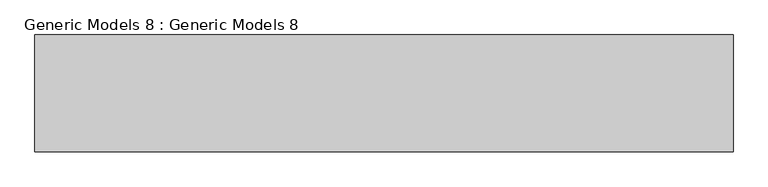
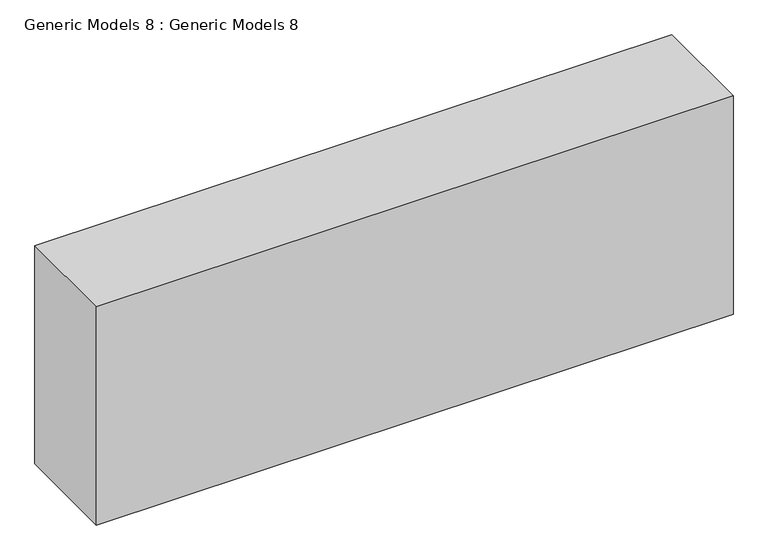
"""IFC4 building model written with IfcOpenShell, lengths in millimetres: proxy geometry, Generic Models 8 : Generic Models 8."""

from ifc_helpers import new_model, si_unit, frame, origin, place, context, project, spatial, polyline, outline, extrude, source, transform, mapped, element, save


def generic_models_8_generic_models_8_410e38da(model_context):
    return source(origin(), model_context, "Body", "SweptSolid", [
        extrude(outline(polyline([(-14730.3406521, -7693.1810793), (-12907.8906521, -7693.1810793), (-12907.8906521, -7997.9810793), (-14730.3406521, -7997.9810793), (-14730.3406521, -7693.1810793)])), frame((0.0, 0.0, 2540.0), z_axis=(0.0, 0.0, 1.0), x_axis=(1.0, 0.0, 0.0)), (0.0, 0.0, 1.0), 660.4),
    ])


if __name__ == "__main__":
    model = new_model("IFC4")
    model_context = context("Model", 3, world=origin())
    ifc_project = project(units=[si_unit("LENGTHUNIT", "METRE", prefix="MILLI")], contexts=[model_context])
    site = spatial("IfcSite", under=ifc_project)
    building = spatial("IfcBuilding", under=site)
    placement = place(None, origin())
    generic_models_8_generic_models_8_shape = generic_models_8_generic_models_8_410e38da(model_context)
    element("IfcBuildingElementProxy", 1, Name="Generic Models 8 : Generic Models 8", ObjectType="Generic Models 8 : Generic Models 8", at=placement, inside=building, context=model_context, shape_type="MappedRepresentation", body=[
        mapped(generic_models_8_generic_models_8_shape, transform((0.0, 0.0, 0.0), x_axis=(1.0, 0.0, 0.0), y_axis=(0.0, 1.0, 0.0), z_axis=(0.0, 0.0, 1.0))),
    ])
    save(model, "model.ifc")

# Revit data of these elements
# Element 1 (IfcBuildingElementProxy, "Generic Models 8 : Generic Models 8")
#   Materials on its faces: "GREY COLOUR FRAME(2)"
# Materials
#   "GREY COLOUR FRAME(2)": class "Generic", colour RGB 120 120 120, transparency 0, Cost = 0
